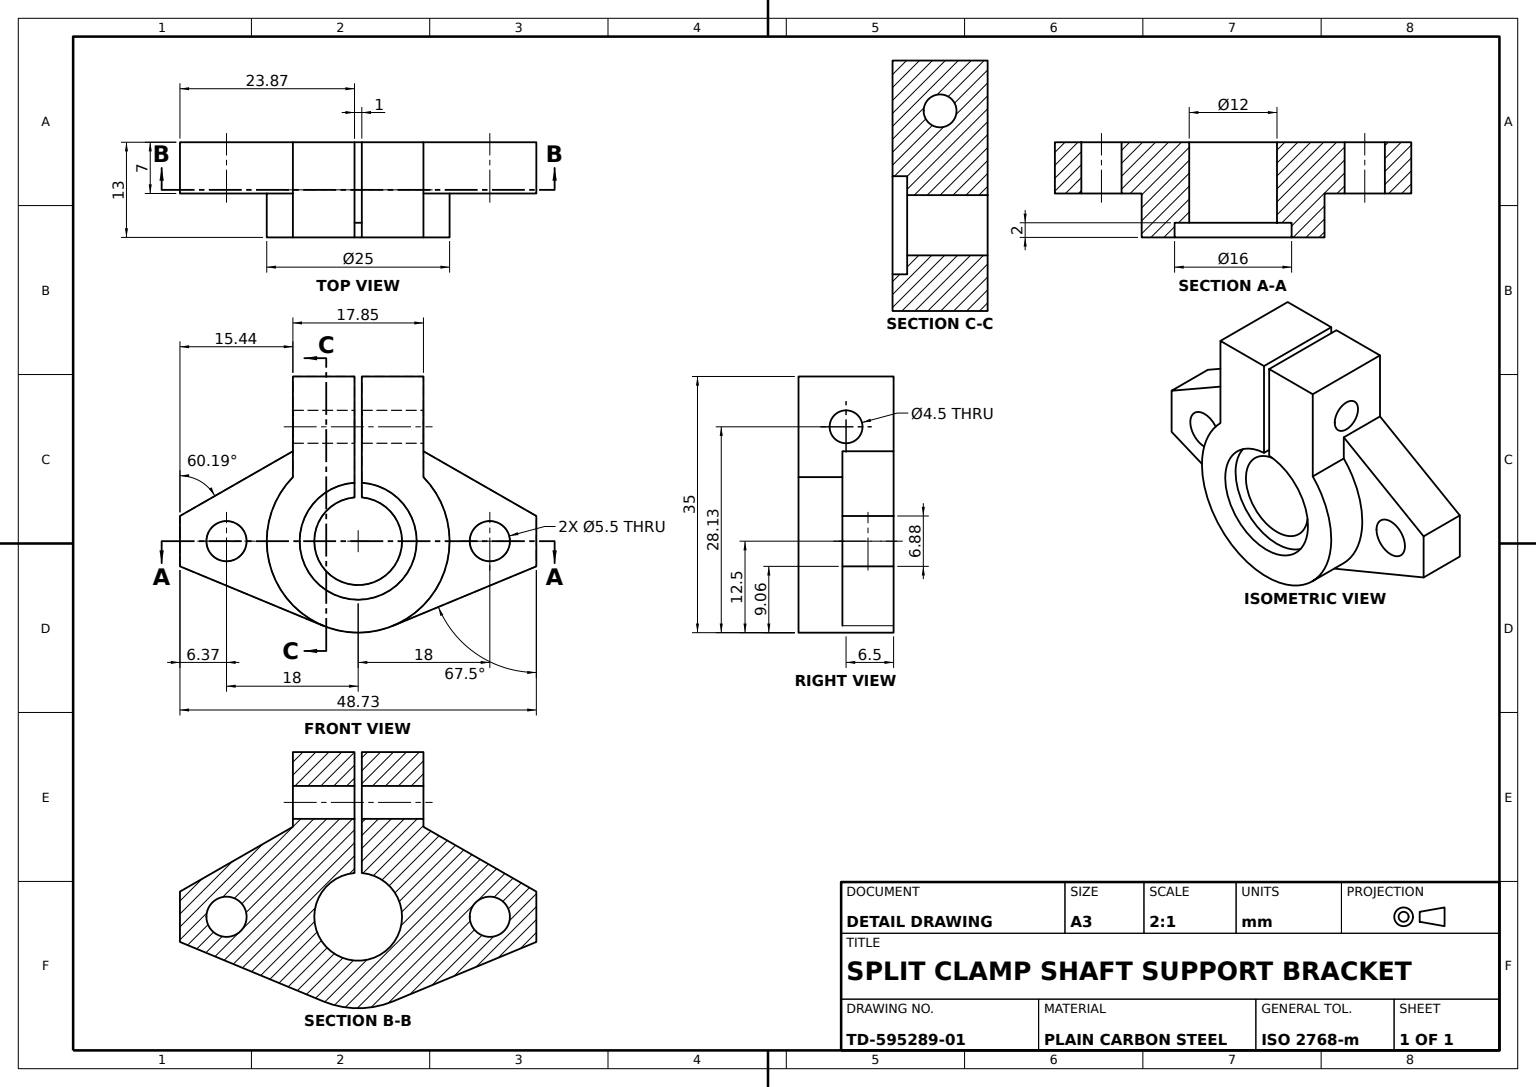
from build123d import *

# Parameters (mm, degrees)
CLAMP_RING_SKETCH_R          = 12.5
CLAMP_RING_25_DEPTH          = 13
CLAMP_BLOCK_DEPTH            = 13
BORE_SKETCH_R                = 6
BORE_12_DEPTH                = 13
COUNTERBORE_SKETCH_R         = 8
COUNTERBORE_16X2_DEPTH       = 2
MOUNTING_FLANGE_SKETCH_R     = 2.75
MOUNTING_FLANGE_2X_5_5_DEPTH = 7
CLAMP_SPLIT_SLOT_DEPTH       = 36.622441552
CLAMP_SCREW_HOLE_SKETCH_R    = 2.25
CLAMP_SCREW_HOLE_4_5_DEPTH   = 20


with BuildPart() as part:
    # Clamp Ring Sketch → Clamp Ring Ø25 (new body)
    with BuildSketch(Plane.XY):
        with Locations(Location((0, 0, 0), (0, 0, 180))):
            Circle(CLAMP_RING_SKETCH_R)
    extrude(amount=CLAMP_RING_25_DEPTH)

    # Clamp Block Sketch → Clamp Block (add)
    with BuildSketch(Plane.XY):
        with BuildLine():
            Line((-8.925, 22.5), (8.925, 22.5))
            Line((8.925, 22.5), (8.925, 8.751821239))
            ThreePointArc((8.925, 8.751821239), (0, 12.5), (-8.925, 8.751821239))
            Line((-8.925, 8.751821239), (-8.925, 22.5))
        make_face()
    extrude(amount=CLAMP_BLOCK_DEPTH)

    # Bore Sketch → Bore Ø12 (cut)
    with BuildSketch(Plane.XY.offset(13)):
        Circle(BORE_SKETCH_R)
    extrude(amount=-BORE_12_DEPTH, mode=Mode.SUBTRACT)

    # Counterbore Sketch → Counterbore Ø16x2 (cut)
    with BuildSketch(Plane.XY.offset(13)):
        Circle(COUNTERBORE_SKETCH_R)
    extrude(amount=-COUNTERBORE_16X2_DEPTH, mode=Mode.SUBTRACT)

    # Mounting Flange Sketch → Mounting Flange 2xØ5.5 (add)
    # profile 1 of 2: a face of its own
    with BuildSketch(Plane.XY):
        with BuildLine():
            Line((-8.925, 12.285952074), (-24.366131046, 3.44))
            Line((-24.366131046, 3.44), (-24.366131046, -3.437120562))
            Line((-24.366131046, -3.437120562), (-4.783542905, -11.548494156))
            ThreePointArc((-4.783542905, -11.548494156), (-12.247723806, -2.498651951), (-8.925, 8.751821239))
            Line((-8.925, 8.751821239), (-8.925, 12.285952074))
        make_face()
        with Locations((-18, 0)):
            Circle(MOUNTING_FLANGE_SKETCH_R, mode=Mode.SUBTRACT)
    # profile 2 of 2: a face of its own
    with BuildSketch(Plane.XY):
        with BuildLine():
            ThreePointArc((8.925, 8.751821239), (12.247723806, -2.498651951), (4.783542905, -11.548494156))
            Line((4.783542905, -11.548494156), (24.359179467, -3.44))
            Line((24.359179467, -3.44), (24.359179467, 3.44))
            Line((24.359179467, 3.44), (8.925, 12.285952074))
            Line((8.925, 12.285952074), (8.925, 8.751821239))
        make_face()
        with Locations((18, 0)):
            Circle(MOUNTING_FLANGE_SKETCH_R, mode=Mode.SUBTRACT)
    extrude(amount=MOUNTING_FLANGE_2X_5_5_DEPTH)

    # Split Slot Sketch → Clamp Split Slot (cut, through all)
    with BuildSketch(Plane.XY.offset(13)):
        with BuildLine():
            Line((0.5, 5.979130372), (0.5, 22.5))
            Line((0.5, 22.5), (-0.5, 22.5))
            Line((-0.5, 22.5), (-0.5, 5.979130372))
            ThreePointArc((-0.5, 5.979130372), (0, 6), (0.5, 5.979130372))
        make_face()
    extrude(amount=-CLAMP_SPLIT_SLOT_DEPTH, mode=Mode.SUBTRACT)

    # Clamp Screw Hole Sketch → Clamp Screw Hole Ø4.5 (cut)
    with BuildSketch(Plane(origin=(8.925, 0, 0), x_dir=(0, 0, -1), z_dir=(1, 0, 0))):
        with Locations((-6.5, 15.62591062)):
            Circle(CLAMP_SCREW_HOLE_SKETCH_R)
    extrude(amount=-CLAMP_SCREW_HOLE_4_5_DEPTH, mode=Mode.SUBTRACT)


solid = part.part
